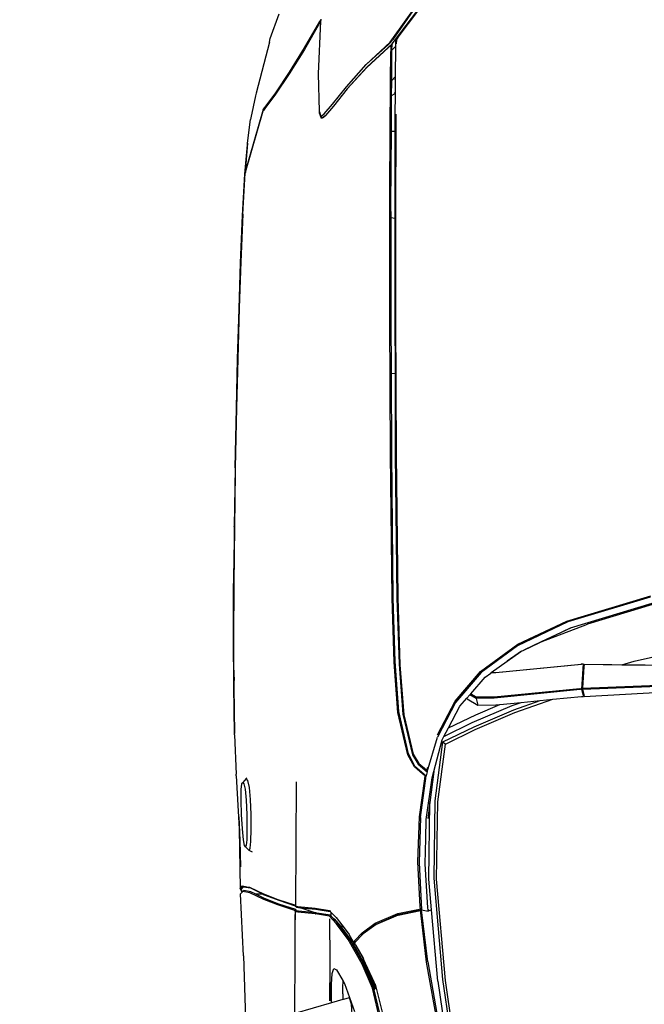
# Model space of a CAD drawing. Units: inches. Extents: x 1319 to 2030, y 219 to 1069.
# Tile 13 of 28: x 1417 to 1444, y 473 to 515. Entities that reach past the tile are written whole.
import ezdxf

# ---------------------------------------------------------------- set-up
doc = ezdxf.new("R2010")
doc.units = ezdxf.units.IN
doc.header["$MEASUREMENT"] = 0
doc.layers.get('0').update_dxf_attribs({"color": 12})
doc.layers.add('A-ANNO-DIMS', color=2, linetype='Continuous', lineweight=18)
doc.layers.add('C-PRKG-VEHC', color=8, linetype='Continuous', lineweight=13)
doc.layers.add('Edges', color=250, linetype='Continuous')
doc.styles.get("Standard").update_dxf_attribs({"font": 'arial.ttf'})
doc.dimstyles.get("Standard").update_dxf_attribs({"dimtxt": 7, "dimasz": 0.18, "dimexe": 0.18, "dimexo": 0.0625, "dimgap": 0.09, "dimtad": 0, "dimtih": 1, "dimtoh": 1, "dimzin": 0, "dimdsep": 46, "dimlunit": 3, "dimtxsty": 'Standard', "dimcen": 0.09, "dimadec": 0, "dimazin": 0, "dimtfac": 1, "dimtofl": 0, "dimtmove": 0, "dimatfit": 3, "dimfxl": 1, "dimtolj": 1, "dimtzin": 0, "dimarcsym": 0})

# ---------------------------------------------------------------- blocks, each defined once
blk = doc.blocks.new('Nissan Qashqai pl')
at = {"layer": 'Edges'}
for p, q in [((8.4086, 11.6764), (8.4045, 11.4011)), ((8.4305, 11.3996), (8.419, 11.6758)), ((8.4204, 11.6758), (8.4319, 11.3996)), ((8.4394, 11.4014), (8.4238, 11.6766)), ((8.4009, 11.4559), (8.3792, 11.5515)), ((8.3573, 11.3824), (8.3296, 11.4739)), ((8.3311, 11.4733), (8.3582, 11.3836)), ((8.3648, 11.3863), (8.3377, 11.4753)), ((8.3392, 11.4758), (8.3608, 11.4048)), ((8.4048, 11.4423), (8.4051, 11.4678)), ((8.4048, 11.4423), (8.4009, 11.4559)), ((8.4041, 11.4013), (8.4048, 11.4423)), ((8.3799, 11.3545), (8.3608, 11.4048)), ((8.407, 11.401), (8.4037, 11.4002)), ((8.4037, 11.4002), (8.4314, 11.3985)), ((8.4037, 11.3992), (8.4037, 11.4002)), ((8.4037, 11.3992), (8.4046, 11.3981)), ((8.4042, 11.3983), (8.4037, 11.3992)), ((8.4041, 11.4013), (8.4045, 11.4011)), ((8.4134, 11.3049), (8.4042, 11.3983)), ((8.4045, 11.4011), (8.407, 11.401)), ((8.4046, 11.3981), (8.4138, 11.3048)), ((8.407, 11.401), (8.4305, 11.3996)), ((8.4305, 11.3996), (8.4319, 11.3996)), ((8.4314, 11.3985), (8.4394, 11.4004)), ((8.4314, 11.3985), (8.4314, 11.3975)), ((8.4319, 11.3996), (8.436, 11.4006)), ((8.436, 11.4006), (8.4394, 11.4014)), ((8.4394, 11.4004), (8.436, 11.4006)), ((8.4394, 11.3984), (8.4394, 11.4004)), ((8.4425, 11.3672), (8.4394, 11.3984)), ((8.4306, 11.3966), (8.4314, 11.3975)), ((8.4398, 11.3032), (8.4306, 11.3966)), ((8.4314, 11.3975), (8.4319, 11.3967)), ((8.4319, 11.3967), (8.4412, 11.3033)), ((8.3826, 11.3291), (8.3573, 11.3824)), ((8.3582, 11.3836), (8.3844, 11.3284)), ((8.3646, 11.387), (8.3799, 11.3545)), ((8.3888, 11.3355), (8.3648, 11.3863)), ((8.4571, 11.3258), (8.4425, 11.3672)), ((8.4439, 11.3531), (8.4425, 11.3672)), ((8.3799, 11.3545), (8.3888, 11.3355)), ((8.454, 11.3245), (8.4439, 11.3531)), ((8.4459, 11.3326), (8.4439, 11.3531)), ((8.3901, 11.3328), (8.3888, 11.3355)), ((8.4122, 11.2883), (8.3826, 11.3291)), ((8.3844, 11.3284), (8.4134, 11.2888)), ((8.3901, 11.3328), (8.4011, 11.3173)), ((8.3904, 11.3321), (8.3901, 11.3328)), ((8.4011, 11.3173), (8.3904, 11.3321)), ((8.4493, 11.3229), (8.4459, 11.3326)), ((8.4482, 11.3095), (8.4459, 11.3326)), ((8.4725, 11.2812), (8.454, 11.3245)), ((8.4756, 11.2826), (8.4571, 11.3258)), ((8.4135, 11.3), (8.4011, 11.3173)), ((8.468, 11.2793), (8.4493, 11.3229)), ((8.4135, 11.3), (8.4134, 11.3049)), ((8.4138, 11.3048), (8.4139, 11.2994)), ((8.44, 11.2834), (8.4398, 11.3032)), ((8.4412, 11.3033), (8.4415, 11.2835)), ((8.4594, 11.2831), (8.4482, 11.3095)), ((8.4487, 11.305), (8.4482, 11.3095)), ((8.4489, 11.2852), (8.4487, 11.305)), ((8.4139, 11.2994), (8.4135, 11.3)), ((8.4183, 11.2934), (8.4139, 11.2994)), ((8.4365, 11.2776), (8.4183, 11.2934)), ((8.4444, 11.2608), (8.4122, 11.2883)), ((8.4134, 11.2888), (8.4462, 11.2609)), ((8.4365, 11.2776), (8.44, 11.2834)), ((8.4415, 11.2835), (8.4375, 11.2767)), ((8.4415, 11.2835), (8.4489, 11.2852)), ((8.4422, 11.2737), (8.4489, 11.2852)), ((8.4737, 11.2534), (8.4594, 11.2831)), ((8.4889, 11.2473), (8.4725, 11.2812)), ((8.4914, 11.25), (8.4756, 11.2826)), ((8.4375, 11.2767), (8.4365, 11.2776)), ((8.4412, 11.2735), (8.4375, 11.2767)), ((8.4422, 11.2737), (8.4412, 11.2735)), ((8.4499, 11.2659), (8.4412, 11.2735)), ((8.4831, 11.2484), (8.468, 11.2793)), ((8.4814, 11.2413), (8.4444, 11.2608)), ((8.4462, 11.2609), (8.4838, 11.2415)), ((8.4737, 11.2534), (8.4499, 11.2659)), ((8.8745, 11.266), (8.7481, 11.2473)), ((8.8754, 11.2687), (8.7491, 11.2501)), ((8.7496, 11.2416), (8.8761, 11.2602)), ((8.4831, 11.2484), (8.4737, 11.2534)), ((8.4867, 11.2465), (8.4831, 11.2484)), ((8.4889, 11.2473), (8.4914, 11.25)), ((8.5544, 11.2416), (8.4914, 11.25)), ((8.7491, 11.2501), (8.6386, 11.2404)), ((8.7287, 11.2307), (8.8666, 11.2554)), ((8.8666, 11.2541), (8.7292, 11.2295)), ((8.5216, 11.2303), (8.4838, 11.2415)), ((8.528, 11.2354), (8.4867, 11.2465)), ((8.5214, 11.2374), (8.4867, 11.2465)), ((8.5531, 11.2387), (8.4889, 11.2473)), ((8.5214, 11.2374), (8.555, 11.233)), ((8.5301, 11.2352), (8.5214, 11.2374)), ((8.6375, 11.2376), (8.5531, 11.2387)), ((8.6386, 11.2404), (8.5544, 11.2416)), ((8.7481, 11.2473), (8.6375, 11.2376)), ((8.7496, 11.2416), (8.6721, 11.2348)), ((7.6769, 11.2312), (7.7194, 11.1992)), ((7.7232, 11.1955), (7.6771, 11.2307)), ((8.5125, 11.221), (8.5177, 11.2272)), ((8.5132, 11.2202), (8.5216, 11.2303)), ((8.5155, 11.2168), (8.5258, 11.2291)), ((8.5197, 11.2297), (8.5166, 11.2307)), ((8.5177, 11.2272), (8.5197, 11.2297)), ((8.5216, 11.2303), (8.5197, 11.2297)), ((8.5216, 11.2303), (8.5258, 11.2291)), ((8.5259, 11.2279), (8.5237, 11.2252)), ((8.5258, 11.2291), (8.5259, 11.2279)), ((8.5715, 11.2227), (8.5258, 11.2291)), ((8.5294, 11.2274), (8.5259, 11.2279)), ((8.5736, 11.2291), (8.528, 11.2354)), ((8.5706, 11.2216), (8.5294, 11.2274)), ((8.6387, 11.2319), (8.555, 11.233)), ((8.555, 11.233), (8.5726, 11.2307)), ((8.5941, 11.2286), (8.5736, 11.2291)), ((8.5941, 11.2289), (8.5941, 11.2286)), ((8.622, 11.228), (8.5941, 11.2286)), ((8.6699, 11.231), (8.622, 11.228)), ((8.6721, 11.2348), (8.6387, 11.2319)), ((8.6721, 11.2312), (8.6699, 11.231)), ((8.6721, 11.2348), (8.6733, 11.2313)), ((8.6721, 11.2312), (8.6721, 11.2318)), ((8.6721, 11.2241), (8.6733, 11.2313)), ((8.6733, 11.2313), (8.6721, 11.2312)), ((8.7287, 11.2307), (8.6721, 11.2241)), ((8.7292, 11.2295), (8.6753, 11.2232)), ((7.7261, 11.1898), (7.6762, 11.2256)), ((7.6762, 11.2256), (7.7233, 11.1928)), ((8.5155, 11.2168), (8.5018, 11.2098)), ((8.5025, 11.2148), (8.5125, 11.221)), ((8.5163, 11.2162), (8.5029, 11.2092)), ((8.5032, 11.2141), (8.5132, 11.2202)), ((8.5237, 11.2252), (8.5163, 11.2162)), ((8.6197, 11.2201), (8.5706, 11.2216)), ((8.5715, 11.2227), (8.6203, 11.2213)), ((8.6683, 11.2226), (8.6197, 11.2201)), ((8.6203, 11.2213), (8.6721, 11.2241)), ((8.671, 11.2227), (8.6683, 11.2226)), ((8.6721, 11.2241), (8.671, 11.2227)), ((8.6716, 11.2199), (8.671, 11.2227)), ((8.6759, 11.1982), (8.6716, 11.2199)), ((8.6721, 11.2241), (8.6727, 11.2229)), ((8.6772, 11.1988), (8.6721, 11.2241)), ((8.6753, 11.2232), (8.6727, 11.2229)), ((8.6777, 11.1984), (8.6727, 11.2229)), ((8.5018, 11.2098), (8.4559, 11.1991)), ((8.5029, 11.2092), (8.4571, 11.1983)), ((8.4588, 11.2036), (8.5032, 11.2141)), ((8.4595, 11.2047), (8.5025, 11.2148)), ((7.7194, 11.1992), (7.7232, 11.1966)), ((7.7232, 11.1966), (7.7279, 11.1965)), ((7.7281, 11.1918), (7.7232, 11.1955)), ((7.7232, 11.1955), (7.7245, 11.1955)), ((7.7247, 11.1954), (7.7245, 11.1955)), ((7.7245, 11.1955), (7.7294, 11.1955)), ((7.7294, 11.1955), (7.731, 11.1955)), ((7.731, 11.1955), (7.7349, 11.1917)), ((7.731, 11.1955), (7.764, 11.1953)), ((7.764, 11.1953), (7.7636, 11.1957)), ((7.768, 11.1915), (7.764, 11.1953)), ((7.764, 11.1953), (7.7662, 11.1953)), ((7.7659, 11.1957), (7.7662, 11.1953)), ((7.7662, 11.1953), (7.7668, 11.1946)), ((7.7662, 11.1953), (7.7811, 11.1952)), ((7.7811, 11.1952), (7.7809, 11.1958)), ((7.7814, 11.1946), (7.7811, 11.1952)), ((7.7811, 11.1952), (7.7822, 11.1952)), ((7.7822, 11.1952), (7.7819, 11.1958)), ((7.7822, 11.1952), (7.8057, 11.195)), ((7.7844, 11.1913), (7.7822, 11.1952)), ((7.8048, 11.1959), (7.8233, 11.1958)), ((7.8057, 11.195), (7.8233, 11.195)), ((7.8233, 11.195), (7.8233, 11.1958)), ((7.8233, 11.1958), (7.9014, 11.1955)), ((7.8233, 11.195), (7.902, 11.1947)), ((7.8233, 11.1911), (7.8233, 11.195)), ((7.9014, 11.1955), (7.9185, 11.1955)), ((7.902, 11.1947), (7.9183, 11.1947)), ((7.9183, 11.1947), (7.9176, 11.1908)), ((7.9185, 11.1955), (7.9183, 11.1947)), ((7.9183, 11.1947), (8.0275, 11.1948)), ((7.9185, 11.1955), (8.0273, 11.1957)), ((8.0273, 11.1957), (8.1753, 11.1963)), ((8.0275, 11.1948), (8.0876, 11.1951)), ((8.0876, 11.1951), (8.0873, 11.1911)), ((8.0876, 11.1951), (8.1754, 11.1954)), ((8.1753, 11.1963), (8.3318, 11.198)), ((8.1754, 11.1954), (8.332, 11.1971)), ((8.3318, 11.198), (8.4049, 11.2004)), ((8.332, 11.1971), (8.4042, 11.1995)), ((8.4014, 11.1953), (8.3324, 11.1931)), ((8.4022, 11.1943), (8.3324, 11.192)), ((8.4559, 11.1991), (8.4014, 11.1953)), ((8.4571, 11.1983), (8.4022, 11.1943)), ((8.4042, 11.1995), (8.4588, 11.2036)), ((8.4049, 11.2004), (8.4595, 11.2047)), ((8.6864, 11.1736), (8.6759, 11.1982)), ((8.6875, 11.1744), (8.6772, 11.1988)), ((8.6777, 11.1984), (8.6883, 11.1737)), ((7.7267, 11.1902), (7.7233, 11.1928)), ((7.7261, 11.1898), (7.7507, 11.1638)), ((7.7286, 11.1881), (7.7267, 11.1902)), ((7.7281, 11.1918), (7.7299, 11.1904)), ((7.7349, 11.1917), (7.7281, 11.1918)), ((7.753, 11.1648), (7.7281, 11.1918)), ((7.7507, 11.1638), (7.7286, 11.1881)), ((7.7299, 11.1904), (7.7324, 11.1876)), ((7.7299, 11.1904), (7.7364, 11.1904)), ((7.7324, 11.1876), (7.7539, 11.1642)), ((7.768, 11.1915), (7.7349, 11.1917)), ((7.7363, 11.1904), (7.7364, 11.1904)), ((7.7694, 11.1901), (7.7364, 11.1904)), ((7.7692, 11.1915), (7.768, 11.1915)), ((7.7694, 11.1901), (7.7687, 11.1908)), ((7.7844, 11.1913), (7.7692, 11.1915)), ((7.7707, 11.1901), (7.7694, 11.1901)), ((7.7851, 11.19), (7.7707, 11.1901)), ((7.8078, 11.1911), (7.7844, 11.1913)), ((7.7846, 11.1909), (7.7851, 11.19)), ((7.8083, 11.1898), (7.7851, 11.19)), ((7.8233, 11.1911), (7.8078, 11.1911)), ((7.904, 11.1894), (7.8083, 11.1898)), ((7.8233, 11.1899), (7.8233, 11.1911)), ((7.9036, 11.1907), (7.8233, 11.1911)), ((7.9176, 11.1908), (7.9036, 11.1907)), ((8.0276, 11.1896), (7.904, 11.1894)), ((8.0275, 11.1909), (7.9176, 11.1908)), ((8.0873, 11.1911), (8.0275, 11.1909)), ((8.1753, 11.1903), (8.0276, 11.1896)), ((8.1755, 11.1915), (8.0873, 11.1911)), ((8.3324, 11.192), (8.1753, 11.1903)), ((8.3324, 11.1931), (8.1755, 11.1915)), ((8.697, 11.1592), (8.6864, 11.1736)), ((8.6979, 11.1603), (8.6875, 11.1744)), ((8.6883, 11.1737), (8.6987, 11.1597)), ((8.7346, 11.1636), (8.7577, 11.1732)), ((8.7491, 11.1703), (8.7576, 11.1743)), ((8.7532, 11.1733), (8.7508, 11.1722)), ((8.7529, 11.17), (8.7577, 11.1732)), ((8.7532, 11.1733), (8.7575, 11.1744)), ((8.7931, 11.1789), (8.7574, 11.1704)), ((8.7575, 11.1744), (8.7881, 11.1821)), ((8.7575, 11.1744), (8.7576, 11.1743)), ((8.7576, 11.1743), (8.7582, 11.1734)), ((8.7577, 11.1732), (8.7582, 11.1734)), ((8.7582, 11.1734), (8.759, 11.1725)), ((8.7925, 11.1802), (8.7591, 11.1723)), ((7.7748, 11.1423), (7.7507, 11.1638)), ((7.753, 11.1648), (7.7772, 11.1431)), ((7.7539, 11.1642), (7.7772, 11.1431)), ((8.7075, 11.1487), (8.7346, 11.1636)), ((8.7508, 11.1722), (8.7257, 11.1609)), ((8.7529, 11.17), (8.7302, 11.1602)), ((8.7574, 11.1704), (8.7312, 11.1591)), ((8.7346, 11.1636), (8.7491, 11.1703)), ((8.7508, 11.1722), (8.7491, 11.1703)), ((8.757, 11.1718), (8.7529, 11.17)), ((8.7587, 11.1722), (8.757, 11.1718)), ((8.759, 11.1725), (8.7587, 11.1722)), ((8.7591, 11.1723), (8.7587, 11.1722)), ((8.759, 11.1725), (8.7591, 11.1723)), ((8.7055, 11.1514), (8.697, 11.1592)), ((8.6987, 11.1596), (8.6979, 11.1603)), ((8.6987, 11.1597), (8.6988, 11.1596)), ((8.6987, 11.1596), (8.6988, 11.1596)), ((8.6996, 11.1588), (8.6987, 11.1596)), ((8.6988, 11.1596), (8.6996, 11.1588)), ((8.6996, 11.1588), (8.6996, 11.1588)), ((8.7062, 11.1527), (8.6996, 11.1588)), ((8.6996, 11.1588), (8.7062, 11.1527)), ((8.7302, 11.1602), (8.7032, 11.145)), ((8.7312, 11.1591), (8.7042, 11.144)), ((8.707, 11.15), (8.7055, 11.1514)), ((8.7067, 11.1522), (8.7062, 11.1527)), ((8.7083, 11.1508), (8.7067, 11.1522)), ((8.7083, 11.1507), (8.7102, 11.1519)), ((8.7102, 11.1519), (8.7108, 11.1523)), ((8.7108, 11.1523), (8.7257, 11.1609)), ((8.7108, 11.1523), (8.7248, 11.1605)), ((8.7248, 11.1605), (8.7257, 11.1609)), ((7.7938, 11.1271), (7.7748, 11.1423)), ((7.7772, 11.1431), (7.7959, 11.1281)), ((8.7042, 11.144), (8.687, 11.131)), ((8.6884, 11.1371), (8.6973, 11.144)), ((8.6917, 11.1371), (8.7075, 11.1487)), ((8.7032, 11.145), (8.6927, 11.1371)), ((8.6973, 11.144), (8.698, 11.1446)), ((8.698, 11.1446), (8.6981, 11.1446)), ((8.7071, 11.15), (8.6981, 11.1446)), ((8.707, 11.15), (8.7083, 11.1508)), ((8.7071, 11.15), (8.707, 11.15)), ((8.707, 11.15), (8.707, 11.15)), ((8.7083, 11.1508), (8.7071, 11.15)), ((8.7083, 11.1508), (8.7083, 11.1507)), ((8.7524, 11.1401), (8.7828, 11.1508)), ((8.7748, 11.1475), (8.7678, 11.1453)), ((8.7678, 11.1453), (8.7698, 11.1385)), ((8.7916, 11.1488), (8.7748, 11.1475)), ((8.6805, 11.1309), (8.6746, 11.1253)), ((8.687, 11.131), (8.6788, 11.1237)), ((8.6805, 11.1309), (8.6884, 11.1371)), ((8.6859, 11.132), (8.6817, 11.1282)), ((8.6818, 11.1288), (8.6902, 11.136)), ((8.6927, 11.1371), (8.6859, 11.132)), ((8.6884, 11.1371), (8.6917, 11.1371)), ((8.6902, 11.136), (8.6917, 11.1371)), ((8.6923, 11.1371), (8.6927, 11.1371)), ((8.7361, 11.1283), (8.7373, 11.1314)), ((8.7373, 11.1314), (8.7492, 11.1383)), ((8.7492, 11.1383), (8.7524, 11.1401)), ((8.7492, 11.1383), (8.7572, 11.1379)), ((8.7572, 11.1379), (8.7698, 11.1383)), ((8.7698, 11.1385), (8.7583, 11.1382)), ((8.7698, 11.1385), (8.7698, 11.1383)), ((8.7698, 11.1383), (8.7733, 11.126)), ((7.8045, 11.1179), (7.7938, 11.1271)), ((7.7959, 11.1281), (7.8062, 11.1192)), ((7.8087, 11.1159), (7.8062, 11.1192)), ((7.8062, 11.1192), (7.8066, 11.1188)), ((8.6703, 11.1081), (8.6727, 11.1235)), ((8.6714, 11.1088), (8.6737, 11.1245)), ((8.6727, 11.1235), (8.6737, 11.1245)), ((8.6737, 11.1245), (8.6746, 11.1253)), ((8.6746, 11.1253), (8.6785, 11.1253)), ((8.6777, 11.1246), (8.6755, 11.1099)), ((8.6788, 11.1237), (8.6764, 11.1083)), ((8.6785, 11.1253), (8.6777, 11.1246)), ((8.6815, 11.128), (8.6785, 11.1253)), ((8.6815, 11.128), (8.6818, 11.1288)), ((8.6817, 11.1282), (8.6815, 11.128)), ((8.6817, 11.1282), (8.6818, 11.1288)), ((8.6818, 11.1238), (8.7026, 11.1238)), ((8.7026, 11.1238), (8.7026, 11.1239)), ((8.7026, 11.1238), (8.7072, 11.1239)), ((8.7072, 11.1239), (8.7072, 11.1239)), ((8.7072, 11.1239), (8.7273, 11.1239)), ((8.7273, 11.1239), (8.7273, 11.124)), ((8.7273, 11.1239), (8.7354, 11.124)), ((8.7354, 11.1241), (8.7354, 11.124)), ((8.7354, 11.124), (8.742, 11.124)), ((8.7415, 11.1265), (8.7361, 11.1283)), ((8.7534, 11.1257), (8.7415, 11.1265)), ((8.742, 11.1241), (8.742, 11.124)), ((8.742, 11.124), (8.742, 11.1241)), ((8.742, 11.124), (8.742, 11.124)), ((8.742, 11.124), (8.7426, 11.124)), ((8.7426, 11.1241), (8.7426, 11.124)), ((8.7426, 11.124), (8.7433, 11.124)), ((8.7433, 11.1241), (8.7433, 11.124)), ((8.7433, 11.124), (8.7711, 11.1241)), ((8.7711, 11.1241), (8.7516, 11.1241)), ((8.7718, 11.126), (8.7534, 11.1257)), ((8.7733, 11.126), (8.7718, 11.126)), ((8.7733, 11.126), (8.7849, 11.0859)), ((7.701, 11.1141), (7.7024, 11.1141)), ((7.7038, 11.1132), (7.7024, 11.1141)), ((7.7024, 11.1141), (7.7034, 11.114)), ((7.7034, 11.114), (7.7056, 11.1128)), ((7.7034, 11.114), (7.7608, 11.1112)), ((7.7325, 11.0966), (7.7038, 11.1132)), ((7.7056, 11.1128), (7.7341, 11.0963)), ((7.7608, 11.1112), (7.8014, 11.1124)), ((7.8014, 11.1124), (7.8022, 11.1126)), ((7.8022, 11.1126), (7.8072, 11.1141)), ((7.8037, 11.1126), (7.8022, 11.1126)), ((7.8096, 11.1148), (7.8037, 11.1126)), ((7.8072, 11.1141), (7.8045, 11.1179)), ((7.8066, 11.1188), (7.8096, 11.1148)), ((7.8072, 11.1141), (7.8087, 11.1159)), ((8.6697, 11.0922), (8.6714, 11.1088)), ((8.6698, 11.0925), (8.6755, 11.1099)), ((8.6754, 11.1089), (8.6735, 11.0898)), ((8.6755, 11.1099), (8.6754, 11.1089)), ((8.6684, 11.0892), (8.6703, 11.1081)), ((8.6764, 11.1082), (8.6744, 11.0891)), ((8.6764, 11.1082), (8.6764, 11.1083)), ((7.7591, 11.08), (7.7325, 11.0966)), ((7.7341, 11.0963), (7.7606, 11.0798)), ((8.5326, 11.0874), (8.6675, 11.0866)), ((8.6682, 11.087), (8.6684, 11.0888)), ((8.6692, 11.0876), (8.6682, 11.0866)), ((8.6682, 11.087), (8.6692, 11.0876)), ((8.6682, 11.0866), (8.6682, 11.087)), ((8.6684, 11.0888), (8.6684, 11.0892)), ((8.6684, 11.0888), (8.6685, 11.089)), ((8.6692, 11.0876), (8.6697, 11.0922)), ((8.6697, 11.0922), (8.6698, 11.0925)), ((8.6729, 11.0874), (8.6718, 11.0868)), ((8.6733, 11.0875), (8.6729, 11.0874)), ((8.6735, 11.0898), (8.6733, 11.0875)), ((8.6744, 11.0891), (8.6742, 11.0866)), ((7.7814, 11.065), (7.7591, 11.08)), ((7.7606, 11.0798), (7.7828, 11.0649)), ((8.6606, 11.0674), (8.6667, 11.0857)), ((8.6616, 11.0683), (8.6675, 11.0862)), ((8.6718, 11.0868), (8.6657, 11.0684)), ((8.6667, 11.0857), (8.6675, 11.0862)), ((8.6728, 11.0858), (8.6667, 11.0675)), ((8.6674, 11.0864), (8.6675, 11.0865)), ((8.6675, 11.0865), (8.6675, 11.0866)), ((8.6676, 11.0866), (8.6675, 11.0866)), ((8.6675, 11.0862), (8.6679, 11.0864)), ((8.6676, 11.0864), (8.6677, 11.0866)), ((8.6677, 11.0866), (8.6676, 11.0866)), ((8.6682, 11.0866), (8.6677, 11.0866)), ((8.6679, 11.0864), (8.6682, 11.0866)), ((8.674, 11.0864), (8.6728, 11.0858)), ((8.6742, 11.0866), (8.674, 11.0864)), ((8.6744, 11.0866), (8.6742, 11.0866)), ((8.6742, 11.0858), (8.6743, 11.086)), ((8.6744, 11.0864), (8.6744, 11.0866)), ((8.6773, 11.0865), (8.6744, 11.0866)), ((8.6791, 11.0864), (8.677, 11.0864)), ((8.6791, 11.0865), (8.6773, 11.0865)), ((8.6791, 11.0865), (8.6791, 11.0864)), ((8.6878, 11.0864), (8.6791, 11.0865)), ((8.7205, 11.0863), (8.6791, 11.0864)), ((8.6878, 11.0864), (8.6791, 11.0864)), ((8.6878, 11.0865), (8.6878, 11.0864)), ((8.6911, 11.0864), (8.6878, 11.0864)), ((8.7205, 11.0863), (8.6911, 11.0864)), ((8.7849, 11.0859), (8.7205, 11.0863)), ((7.7223, 11.059), (7.6953, 11.0688)), ((8.6546, 11.0516), (8.6606, 11.0674)), ((8.6556, 11.0524), (8.6616, 11.0683)), ((8.6657, 11.0684), (8.6598, 11.0529)), ((8.6667, 11.0675), (8.6608, 11.0521)), ((7.7262, 11.0581), (7.7223, 11.059)), ((7.7262, 11.0581), (7.7819, 11.0438)), ((7.797, 11.0534), (7.7814, 11.065)), ((7.7828, 11.0649), (7.7984, 11.0533)), ((7.797, 11.0534), (7.797, 11.0534)), ((7.7998, 11.0513), (7.797, 11.0534)), ((7.7984, 11.0533), (7.8007, 11.0516)), ((7.7998, 11.0513), (7.8676, 11.0318)), ((7.8007, 11.0516), (7.8002, 11.0517)), ((7.8007, 11.0516), (7.8012, 11.0513)), ((7.8681, 11.032), (7.8012, 11.0513)), ((8.6472, 11.0366), (8.6546, 11.0516)), ((8.6482, 11.0375), (8.655, 11.0513)), ((8.6608, 11.0521), (8.6534, 11.0369)), ((8.6598, 11.0529), (8.655, 11.0432)), ((8.655, 11.0513), (8.6556, 11.0524)), ((8.655, 11.0513), (8.655, 11.0432)), ((7.7819, 11.0438), (7.7848, 11.043)), ((7.7848, 11.043), (7.8087, 11.038)), ((7.8087, 11.038), (7.8106, 11.0377)), ((7.8107, 11.0377), (7.8106, 11.0377)), ((7.8363, 11.0344), (7.8107, 11.0377)), ((7.8381, 11.0342), (7.8363, 11.0344)), ((7.8363, 11.0344), (7.8676, 11.0318)), ((7.87, 11.0315), (7.8381, 11.0342)), ((8.5283, 11.0336), (8.5287, 11.0329)), ((8.531, 11.0346), (8.5287, 11.0329)), ((8.5385, 11.0363), (8.531, 11.0346)), ((8.5518, 11.0375), (8.5385, 11.0363)), ((8.568, 11.0382), (8.5518, 11.0375)), ((8.5526, 11.0328), (8.5681, 11.0335)), ((8.5842, 11.0384), (8.568, 11.0382)), ((8.5681, 11.0335), (8.5836, 11.0337)), ((8.5836, 11.0337), (8.5957, 11.0334)), ((8.5974, 11.0381), (8.5842, 11.0384)), ((8.5957, 11.0334), (8.6017, 11.0328)), ((8.6049, 11.0373), (8.5974, 11.0381)), ((8.6073, 11.0362), (8.6032, 11.0321)), ((8.6073, 11.0362), (8.6049, 11.0373)), ((8.609, 11.0397), (8.6073, 11.0362)), ((8.646, 11.0289), (8.6468, 11.0337)), ((8.6468, 11.0337), (8.6472, 11.0366)), ((8.647, 11.03), (8.6468, 11.0337)), ((8.647, 11.03), (8.6482, 11.0375)), ((8.6524, 11.0378), (8.651, 11.0302)), ((8.6534, 11.0369), (8.652, 11.0292)), ((8.655, 11.0432), (8.6524, 11.0378)), ((7.8681, 11.032), (7.8676, 11.0318)), ((7.8681, 11.032), (7.869, 11.0317)), ((7.9137, 11.0292), (7.869, 11.0317)), ((7.9151, 11.029), (7.87, 11.0315)), ((7.9137, 11.0292), (7.9658, 11.027)), ((7.9668, 11.0268), (7.9151, 11.029)), ((7.9658, 11.027), (8.016, 11.0253)), ((8.0168, 11.0251), (7.9668, 11.0268)), ((8.016, 11.0253), (8.0713, 11.0237)), ((8.0718, 11.0235), (8.0168, 11.0251)), ((8.0713, 11.0237), (8.1249, 11.0223)), ((8.1251, 11.0222), (8.0718, 11.0235)), ((8.5259, 11.0221), (8.5838, 11.0251)), ((8.5287, 11.0329), (8.5331, 11.0292)), ((8.5331, 11.0292), (8.5346, 11.0303)), ((8.5347, 11.0282), (8.5331, 11.0292)), ((8.5346, 11.0303), (8.5406, 11.0316)), ((8.5407, 11.0274), (8.5347, 11.0282)), ((8.5406, 11.0316), (8.5526, 11.0328)), ((8.5527, 11.0273), (8.5407, 11.0274)), ((8.5682, 11.0278), (8.5527, 11.0273)), ((8.5837, 11.0288), (8.5682, 11.0278)), ((8.5707, 11.0248), (8.5965, 11.0258)), ((8.5958, 11.0301), (8.5837, 11.0288)), ((8.5838, 11.0251), (8.6489, 11.0263)), ((8.5838, 11.0251), (8.5965, 11.0258)), ((8.6018, 11.0312), (8.5958, 11.0301)), ((8.5965, 11.0258), (8.6252, 11.0268)), ((8.6017, 11.0328), (8.6032, 11.0321)), ((8.6032, 11.0321), (8.6018, 11.0312)), ((8.6489, 11.0263), (8.646, 11.0289)), ((8.6498, 11.0273), (8.647, 11.03)), ((8.6527, 11.0286), (8.6489, 11.0263)), ((8.6524, 11.0289), (8.6498, 11.0273)), ((8.651, 11.0302), (8.652, 11.0292)), ((8.652, 11.0292), (8.6524, 11.0289)), ((8.6524, 11.0289), (8.6527, 11.0286)), ((8.6527, 11.0286), (8.6537, 11.0275)), ((8.6547, 11.0265), (8.6537, 11.0275)), ((8.6537, 11.0275), (8.6537, 11.0275)), ((8.7222, 11.0298), (8.6547, 11.0265)), ((8.7222, 11.0298), (8.7908, 11.0322)), ((8.1249, 11.0223), (8.1901, 11.021)), ((8.1902, 11.0208), (8.1251, 11.0222)), ((8.1901, 11.021), (8.1938, 11.021)), ((8.1902, 11.021), (8.1938, 11.021)), ((8.1904, 11.0209), (8.1902, 11.0208)), ((8.1904, 11.0209), (8.2543, 11.0198)), ((8.1938, 11.021), (8.1954, 11.0209)), ((8.1954, 11.0209), (8.2544, 11.02)), ((8.2544, 11.0198), (8.2543, 11.0199)), ((8.2543, 11.0198), (8.2544, 11.0198)), ((8.2544, 11.02), (8.3166, 11.0193)), ((8.2544, 11.0198), (8.2556, 11.0198)), ((8.2556, 11.0198), (8.256, 11.0198)), ((8.256, 11.0198), (8.2561, 11.0198)), ((8.2561, 11.0198), (8.2693, 11.0197)), ((8.2693, 11.0197), (8.2694, 11.0197)), ((8.2694, 11.0197), (8.3098, 11.0192)), ((8.3098, 11.0192), (8.3163, 11.0192)), ((8.3663, 11.019), (8.3163, 11.0192)), ((8.3597, 11.019), (8.3163, 11.0192)), ((8.3166, 11.0193), (8.3764, 11.0191)), ((8.3602, 11.019), (8.3597, 11.019)), ((8.3608, 11.019), (8.3602, 11.019)), ((8.3663, 11.019), (8.3608, 11.019)), ((8.3663, 11.019), (8.3764, 11.0191)), ((8.3757, 11.019), (8.3663, 11.019)), ((8.4282, 11.0193), (8.3757, 11.019)), ((8.3764, 11.0191), (8.4069, 11.0192)), ((8.4069, 11.0192), (8.4219, 11.0196)), ((8.4069, 11.0192), (8.4292, 11.0193)), ((8.4799, 11.0202), (8.4282, 11.0193)), ((8.4292, 11.0193), (8.4799, 11.0202)), ((8.4811, 11.0203), (8.4799, 11.0202)), ((8.4811, 11.0203), (8.5241, 11.022)), ((8.5259, 11.0221), (8.5241, 11.022))]:
    blk.add_line(p, q, dxfattribs=at)
blk = doc.blocks.new('car')
blk.add_blockref('Nissan Qashqai pl', (-9.7433, -11.9151))
blk = doc.blocks.new('carr')
blk.add_blockref('car', (0.5124, -0.007))
blk = doc.blocks.new('*D56')
at = {"layer": 'A-ANNO-DIMS', "color": 0, "lineweight": -2, "transparency": 16777216}
for p, q in [((1419.852, 531.201), (1393.865, 531.201)), ((1394.045, 531.021), (1394.045, 448.679)), ((1394.045, 358.918), (1394.045, 441.26)), ((1419.852, 358.738), (1393.865, 358.738))]:
    blk.add_line(p, q, dxfattribs=at)
at = {"layer": 'A-ANNO-DIMS', "color": 0, "transparency": 16777216}
for points in [[(1394.015, 531.021), (1394.075, 531.021), (1394.045, 531.201)], [(1394.015, 358.918), (1394.075, 358.918), (1394.045, 358.738)]]:
    blk.add_solid(points, dxfattribs=at)
at = {"layer": 'Defpoints', "color": 0, "transparency": 16777216}
for p in [(1419.914, 531.201), (1394.045, 358.738), (1419.914, 358.738)]:
    blk.add_point(p, dxfattribs=at)
at = {"layer": 'A-ANNO-DIMS', "color": 0, "transparency": 16777216, "insert": (1394.045, 444.969), "char_height": 7, "attachment_point": 5}
blk.add_mtext('\\A1;CAR 14\'-4 1/2"', dxfattribs=at)

msp = doc.modelspace()

# ---------------------------------------------------------------- block references
at = {"layer": 'C-PRKG-VEHC', "xscale": 39.37007874015748, "yscale": 39.37007874015748, "zscale": 39.37007874015748, "rotation": 270}
msp.add_blockref('carr', (1462.179, 454.621), dxfattribs=at)

# ---------------------------------------------------------------- dimensions: what is measured, and where the dimension line sits
at = {"layer": 'A-ANNO-DIMS'}
dim = msp.add_linear_dim(base=(1394.045, 358.738), p1=(1419.914, 531.201), p2=(1419.914, 358.738), angle=270, text='CAR <>', dimstyle='Standard', override={"dimdec": 1, "dimlfac": 1, "dimrnd": 0, "dimzin": 1, "dimdsep": 46, "dimlunit": 4, "dimfrac": 2}, dxfattribs=at)
dim.commit()
dim.dimension.update_dxf_attribs({"geometry": '*D56', "text_midpoint": (1394.045, 444.969)})

doc.saveas('drawing.dxf')
